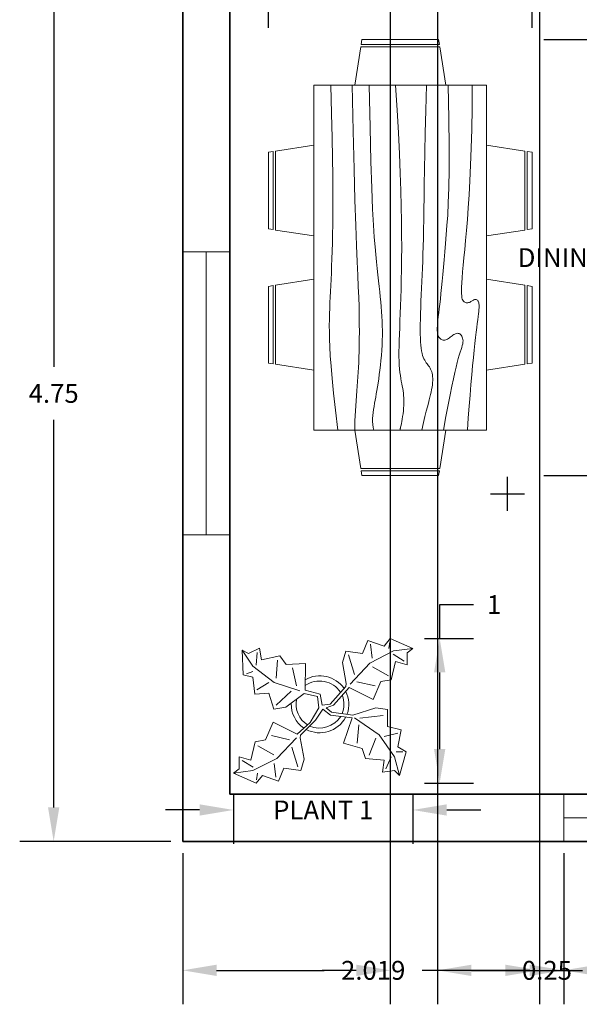
# Model space of a CAD drawing. Units: metres. Extents: x 180.3 to 196.1, y 135.7 to 166.1.
# Tile 1 of 5: x 180.3 to 183.3, y 150.9 to 156.1. Entities that reach past the tile are written whole.
import ezdxf

# ---------------------------------------------------------------- set-up
doc = ezdxf.new("R2010")
doc.units = ezdxf.units.M
doc.header["$MEASUREMENT"] = 0
for name, color, linetype, lineweight in [('A-ANNO-DIMS', 2, 'Continuous', 18), ('A-FURN', 190, 'Continuous', 18), ('A-GLAZ', 130, 'Continuous', 18), ('wall', 50, 'Continuous', 35)]:
    doc.layers.add(name, color=color, linetype=linetype, lineweight=lineweight)
doc.styles.get("Standard").update_dxf_attribs({"font": 'arial.ttf', "height": 0.1})
doc.dimstyles.get("Standard").update_dxf_attribs({"dimtxt": 0.18, "dimasz": 0.18, "dimexe": 0.18, "dimexo": 0.0625, "dimgap": 0.09, "dimtad": 0, "dimtih": 1, "dimtoh": 1, "dimdec": 4, "dimzin": 0, "dimdsep": 46, "dimtxsty": 'Standard', "dimcen": 0.09, "dimadec": 0, "dimazin": 0, "dimtfac": 1, "dimtdec": 4, "dimtofl": 0, "dimtmove": 0, "dimatfit": 3, "dimfxl": 1, "dimtolj": 1, "dimtzin": 0, "dimarcsym": 0})

# ---------------------------------------------------------------- blocks, each defined once
blk = doc.blocks.new('Dining Set - 36 x 72 in.')
for p, q in [((-22, 27.5), (-22.1562, 26.50042)), ((-22, 27.5), (-6, 27.5)), ((-5.8437, 26.49966), (-6, 27.5)), ((6, 27.5), (5.8438, 26.50042)), ((6, 27.5), (22, 27.5)), ((22.1563, 26.49966), (22, 27.5)), ((-22.2343, 26.00059), (-23.4847, 17.99762)), ((-22.2304, 26), (-5.7608, 26)), ((-5.8416, 26.5), (-22.1534, 26.5)), ((-4.5152, 17.99762), (-5.7655, 25.99926)), ((5.7657, 26.00059), (4.5153, 17.99762)), ((5.7696, 26), (22.2392, 26)), ((22.1584, 26.5), (5.8466, 26.5)), ((23.4848, 17.99762), (22.2345, 25.99926)), ((36, 18), (-36, 18)), ((-36, 18), (-36, -18)), ((36, -18), (36, 18)), ((-44.0006, 8.23428), (-35.9976, 9.48474)), ((-44, 8.23041), (-44, -8.23915)), ((44.0006, 8.23428), (35.9976, 9.48474)), ((44, 8.23041), (44, -8.23915)), ((-45.5, 8), (-44.5004, 8.15617)), ((-45.5, 8), (-45.5, -8)), ((-44.5, -8.15843), (-44.5, 8.15338)), ((44.5, -8.15843), (44.5, 8.15338)), ((45.5, 8), (44.5005, 8.15617)), ((45.5, 8), (45.5, -8)), ((-44.4997, -8.15631), (-45.5, -8)), ((44.4997, -8.15631), (45.5, -8)), ((-35.9976, -9.48476), (-43.9993, -8.2345)), ((35.9976, -9.48476), (43.9993, -8.2345)), ((-36, -18), (36, -18)), ((-22.2343, -26.0006), (-23.4847, -17.99762)), ((-4.5152, -17.99762), (-5.7655, -25.99928)), ((5.7657, -26.0006), (4.5153, -17.99762)), ((23.4848, -17.99762), (22.2345, -25.99928)), ((-22.2304, -26), (-5.7608, -26)), ((-22, -27.5), (-22.1562, -26.50044)), ((-5.8416, -26.5), (-22.1534, -26.5)), ((-5.8437, -26.49967), (-6, -27.5)), ((5.7696, -26), (22.2392, -26)), ((6, -27.5), (5.8438, -26.50044)), ((22.1584, -26.5), (5.8466, -26.5)), ((22.1563, -26.49967), (22, -27.5)), ((-22, -27.5), (-6, -27.5)), ((6, -27.5), (22, -27.5))]:
    blk.add_line(p, q)
for points in [[(-36, 15), (-31.1772, 14.97754), (-26.8079, 14.91406), (-22.8538, 14.81543), (-19.276, 14.6875), (-16.0362, 14.53613), (-13.0957, 14.36718), (-10.4159, 14.18652), (-7.9583, 14), (-5.6904, 13.81315), (-3.6035, 13.63021), (-1.6954, 13.45508), (0.0365, 13.29166), (1.5945, 13.14388), (2.9811, 13.01562), (4.1988, 12.9108), (5.25, 12.83333), (6.1393, 12.78613), (6.8802, 12.76823), (7.4883, 12.77767), (7.9792, 12.8125), (8.3685, 12.87077), (8.6719, 12.95052), (8.9049, 13.0498), (9.0833, 13.16666), (9.2205, 13.29899), (9.3216, 13.44401), (9.3895, 13.59879), (9.4271, 13.76041), (9.4373, 13.92594), (9.4232, 14.09245), (9.3875, 14.257), (9.3333, 14.41666), (9.2638, 14.56917), (9.1836, 14.71484), (9.0975, 14.85465), (9.0104, 14.98958), (8.9272, 15.1206), (8.8529, 15.2487), (8.7922, 15.37483), (8.75, 15.5), (8.7305, 15.62467), (8.7344, 15.74739), (8.7617, 15.86621), (8.8125, 15.97916), (8.8867, 16.08431), (8.9844, 16.17968), (9.1055, 16.26334), (9.25, 16.33333), (9.4189, 16.38802), (9.6172, 16.42708), (9.8506, 16.45052), (10.125, 16.45833), (10.4463, 16.45052), (10.8203, 16.42708), (11.2529, 16.38802), (11.75, 16.33333), (12.3184, 16.26318), (12.9694, 16.17838), (13.7151, 16.07991), (14.5677, 15.96875), (15.5395, 15.84586), (16.6426, 15.71224), (17.8893, 15.56884), (19.2917, 15.41666), (20.859, 15.25667), (22.5879, 15.08984), (24.4721, 14.91715), (26.5052, 14.73958), (28.6809, 14.5581), (30.9929, 14.3737), (33.4347, 14.18733), (36, 14)], [(-36, 10), (-28.9766, 10.14274), (-23.1725, 10.20442), (-18.4241, 10.19775), (-14.5677, 10.13541), (-11.4399, 10.03011), (-8.877, 9.89453), (-6.7154, 9.74137), (-4.7917, 9.58333), (-2.9698, 9.43082), (-1.2246, 9.28515), (0.4415, 9.14534), (2.026, 9.01041), (3.5266, 8.87939), (4.9408, 8.7513), (6.266, 8.62516), (7.5, 8.5), (8.6411, 8.37549), (9.6914, 8.2539), (10.6538, 8.13818), (11.5312, 8.03125), (12.3267, 7.93603), (13.043, 7.85547), (13.6831, 7.79248), (14.25, 7.75), (14.7471, 7.7303), (15.1797, 7.73307), (15.5537, 7.75732), (15.875, 7.80208), (16.1494, 7.86637), (16.3828, 7.94922), (16.5811, 8.04964), (16.75, 8.16666), (16.8944, 8.29915), (17.0143, 8.44531), (17.1089, 8.60319), (17.1771, 8.77083), (17.218, 8.94629), (17.2305, 9.1276), (17.2137, 9.31282), (17.1667, 9.5), (17.0895, 9.6875), (16.987, 9.875), (16.8649, 10.0625), (16.7292, 10.25), (16.5856, 10.4375), (16.4401, 10.625), (16.2985, 10.8125), (16.1667, 11), (16.05, 11.18733), (15.9518, 11.3737), (15.8752, 11.5581), (15.8229, 11.73958), (15.798, 11.91715), (15.8034, 12.08984), (15.842, 12.25667), (15.9167, 12.41666), (16.0295, 12.56836), (16.1784, 12.70833), (16.3605, 12.83268), (16.5729, 12.9375), (16.8127, 13.01888), (17.0768, 13.07291), (17.3625, 13.0957), (17.6667, 13.08333), (17.9894, 13.03312), (18.3418, 12.94726), (18.7382, 12.82918), (19.1927, 12.68229), (19.7195, 12.51001), (20.3327, 12.31575), (21.0465, 12.10294), (21.875, 11.875), (22.8357, 11.63354), (23.959, 11.37304), (25.2786, 11.08618), (26.8282, 10.76562), (28.6414, 10.40405), (30.752, 9.99414), (33.1936, 9.52856), (36, 9)], [(-36, 5.5), (-30.7157, 5.3348), (-26.069, 5.20963), (-21.9946, 5.11767), (-18.4271, 5.05208), (-15.3009, 5.00602), (-12.5508, 4.97265), (-10.1112, 4.94515), (-7.9167, 4.91666), (-5.909, 4.88167), (-4.0586, 4.83984), (-2.3429, 4.79215), (-0.7396, 4.73958), (0.7739, 4.6831), (2.22, 4.6237), (3.6213, 4.56233), (5, 4.5), (6.373, 4.43782), (7.7344, 4.3776), (9.0723, 4.32129), (10.375, 4.27083), (11.6309, 4.22819), (12.8281, 4.19531), (13.9551, 4.17415), (15, 4.16666), (15.954, 4.17448), (16.819, 4.19791), (17.6001, 4.23698), (18.3021, 4.29166), (18.9299, 4.36198), (19.4883, 4.44791), (19.9823, 4.54948), (20.4167, 4.66666), (20.7969, 4.79899), (21.1302, 4.94401), (21.4245, 5.09879), (21.6875, 5.26041), (21.9271, 5.42594), (22.1511, 5.59245), (22.3672, 5.757), (22.5834, 5.91666), (22.8065, 6.06868), (23.0404, 6.21093), (23.2879, 6.34147), (23.5521, 6.45833), (23.8358, 6.55957), (24.142, 6.64323), (24.4735, 6.70735), (24.8334, 6.75), (25.2235, 6.76969), (25.642, 6.76692), (26.0858, 6.74267), (26.5521, 6.69791), (27.0379, 6.63362), (27.5404, 6.55078), (28.0565, 6.45036), (28.5834, 6.33333), (29.1242, 6.19987), (29.7071, 6.04687), (30.3661, 5.87044), (31.1354, 5.66666), (32.0493, 5.43164), (33.142, 5.16146), (34.4475, 4.85221), (36, 4.5)], [(-36, -1), (-30.7915, -0.6591), (-26.0195, -0.38216), (-21.6519, -0.16284), (-17.6563, 0.00521), (-14.0005, 0.12833), (-10.6523, 0.21289), (-7.5796, 0.26522), (-4.75, 0.29166), (-2.134, 0.29793), (0.2878, 0.28711), (2.5317, 0.26163), (4.6146, 0.22396), (6.5529, 0.17651), (8.3633, 0.12174), (10.0623, 0.06209), (11.6667, 0), (13.1899, -0.06201), (14.6341, -0.1211), (15.9982, -0.17432), (17.2813, -0.21875), (18.4823, -0.25147), (19.6003, -0.26953), (20.6343, -0.27002), (21.5834, -0.25), (22.4481, -0.20768), (23.2357, -0.14584), (23.9549, -0.06836), (24.6146, 0.02083), (25.2235, 0.11784), (25.7904, 0.21875), (26.3241, 0.31966), (26.8334, 0.41666), (27.3265, 0.50618), (27.8099, 0.58593), (28.2894, 0.65397), (28.7709, 0.70833), (29.2601, 0.74707), (29.763, 0.76823), (30.2855, 0.76985), (30.8334, 0.75), (31.4088, 0.70784), (31.9994, 0.64713), (32.589, 0.57275), (33.1615, 0.48958), (33.7008, 0.4025), (34.1908, 0.3164), (34.6153, 0.23616), (34.9584, 0.16666), (35.2099, 0.11165), (35.3848, 0.07031), (35.504, 0.04069), (35.5886, 0.02083), (35.6594, 0.00879), (35.7377, 0.0026), (35.8442, 0.00032), (36, 0)], [(-36, -6.5), (-27.1843, -6.31267), (-20.084, -6.1263), (-14.469, -5.9419), (-10.1094, -5.76042), (-6.7752, -5.58285), (-4.2363, -5.41016), (-2.2629, -5.24333), (-0.625, -5.08334), (0.8708, -4.93099), (2.2715, -4.78646), (3.5872, -4.64974), (4.8281, -4.52084), (6.0046, -4.39974), (7.127, -4.28646), (8.2053, -4.18099), (9.25, -4.08334), (10.2705, -3.99382), (11.2734, -3.91407), (12.2647, -3.84603), (13.25, -3.79167), (14.2354, -3.75293), (15.2266, -3.73177), (16.2295, -3.73015), (17.25, -3.75), (18.2912, -3.79248), (19.3451, -3.85547), (20.4009, -3.93604), (21.4479, -4.03125), (22.4754, -4.13819), (23.4727, -4.25391), (24.4289, -4.37549), (25.3334, -4.5), (26.1785, -4.62492), (26.9694, -4.74935), (27.7145, -4.87281), (28.4219, -4.99479), (29.1, -5.11483), (29.7572, -5.23242), (30.4016, -5.34709), (31.0417, -5.45834), (31.6837, -5.56437), (32.3262, -5.65821), (32.9658, -5.73153), (33.599, -5.77604), (34.2224, -5.78345), (34.8327, -5.74545), (35.4264, -5.65373), (36, -5.5)], [(-36, -10), (-26.4022, -9.81299), (-18.4675, -9.62891), (-11.9839, -9.45069), (-6.7396, -9.28125), (-2.5226, -9.12354), (0.8789, -8.98047), (3.6769, -8.85498), (6.0833, -8.75), (8.2767, -8.66765), (10.3021, -8.60677), (12.1712, -8.56543), (13.8958, -8.54167), (15.4876, -8.53353), (16.9583, -8.53907), (18.3197, -8.55632), (19.5834, -8.58334), (20.7616, -8.61841), (21.8685, -8.66081), (22.9188, -8.71004), (23.9271, -8.76563), (24.9081, -8.82707), (25.8763, -8.89388), (26.8465, -8.96558), (27.8334, -9.04167), (28.8474, -9.12118), (29.8828, -9.20117), (30.93, -9.27824), (31.9792, -9.34896), (33.0205, -9.40991), (34.0443, -9.45768), (35.0407, -9.48885), (36, -9.5)], [(-36, -14.5), (-30.0881, -14.33513), (-25.0332, -14.21224), (-20.7312, -14.12647), (-17.0781, -14.07292), (-13.97, -14.04671), (-11.3027, -14.04297), (-8.9724, -14.05681), (-6.875, -14.08334), (-4.9224, -14.11833), (-3.0905, -14.16016), (-1.3709, -14.20785), (0.2448, -14.26042), (1.7647, -14.3169), (3.1973, -14.3763), (4.5507, -14.43767), (5.8333, -14.5), (7.0554, -14.5621), (8.235, -14.62175), (9.3922, -14.67652), (10.5469, -14.72396), (11.7192, -14.76164), (12.929, -14.78711), (14.1965, -14.79794), (15.5417, -14.79167), (16.9933, -14.76424), (18.6152, -14.70508), (20.4804, -14.60197), (22.6615, -14.44271), (25.2312, -14.21509), (28.2624, -13.9069), (31.8277, -13.50594), (36, -13)]]:
    blk.add_lwpolyline(points)
blk = doc.blocks.new('Plant - Rubber or Philodendron')
for p, q in [((8.8871, 10.7908), (9.9809, 13.4933)), ((9.9809, 13.4933), (13.3837, 12.301)), ((10.5828, 12.6946), (10.8893, 9.7953)), ((13.3837, 12.301), (14.68, 13.9039)), ((14.5816, 13.2037), (14.3848, 11.8033)), ((14.68, 13.9039), (19.3848, 11.8146)), ((-16.2005, 11.4774), (-13.9899, 8.1064)), ((-16.2005, 11.4774), (-14.8639, 10.7964)), ((-16.0159, 6.3329), (-16.2005, 11.4774)), ((-14.8639, 10.7964), (-12.6195, 11.8975)), ((-13.3174, 8.325), (-13.0735, 11.0065)), ((-12.6195, 11.8975), (-12.1909, 9.4345)), ((-12.1909, 9.4345), (-8.3829, 10.3)), ((-8.3829, 10.3), (-7.0549, 8.501)), ((4.6914, 8.8812), (5.3859, 11.2828)), ((5.3859, 11.2828), (8.8871, 10.7908)), ((5.9878, 10.4842), (7.1971, 6.3869)), ((15.3859, 11.3055), (10.3916, 8.7942)), ((15.2875, 10.6053), (17.5907, 9.2105)), ((19.3848, 11.8146), (15.3859, 11.3055)), ((19.3848, 11.8146), (18.1868, 10.9119)), ((18.1868, 10.9119), (18.1925, 8.4119)), ((-8.8369, 9.409), (-9.0894, 5.6095)), ((-7.0549, 8.501), (-3.0284, 8.6941)), ((-3.0284, 8.6941), (-3.0709, 3.1041)), ((4.6914, 8.8812), (5.5014, 4.4831)), ((10.3916, 8.7942), (6.2847, 4.4028)), ((15.7909, 9.1065), (14.8995, 5.3044)), ((18.1925, 8.4119), (15.7909, 9.1065)), ((-14.0069, 5.8704), (-16.0159, 6.3329)), ((-15.3434, 6.5514), (-13.9984, 6.9884)), ((-13.9899, 8.1064), (-9.5434, 4.7185)), ((-4.8529, 4.012), (-5.7184, 7.82)), ((14.2977, 6.1031), (10.9934, 7.9956)), ((-13.5868, 2.2894), (-14.0069, 5.8704)), ((-13.1329, 3.1804), (-10.6614, 4.727)), ((-9.5434, 4.7185), (-4.1917, 2.9888)), ((5.4346, 3.9146), (5.5014, 4.4831)), ((7.7005, 4.8881), (11.5025, 3.9967)), ((12.7005, 4.8994), (11.1089, 1.1958)), ((14.8995, 5.3044), (12.7005, 4.8994)), ((-10.6784, 2.491), (-13.5868, 2.2894)), ((-9.5858, -0.8715), (-10.6784, 2.491)), ((-9.1318, 0.0195), (-5.9793, 2.9025)), ((-7.1228, -0.443), (-3.5248, 2.2131)), ((-3.5248, 2.2131), (-3.3011, 2.4355)), ((-3.3011, 2.4355), (-0.5306, 1.7947)), ((-3.0709, 3.1041), (0.0797, 2.3163)), ((0.0797, 2.3163), (0.4866, -0.031)), ((2.1141, 0.2298), (5.4346, 3.9146)), ((6.1032, 3.6844), (2.8262, -0.031)), ((11.1089, 1.1958), (6.1032, 3.6844)), ((-0.5306, 1.7947), (-0.2255, -0.5527)), ((-0.5306, 1.7947), (-0.5306, 1.7947)), ((0.4866, -0.031), (2.1141, 0.2298)), ((-7.1228, -0.443), (-9.5858, -0.8715)), ((-2.019, -3.6148), (-0.2255, -0.5527)), ((-0.9375, -3.1608), (0.5883, -0.8135)), ((0.5883, -0.8135), (2.2447, -2.0916)), ((2.8262, -0.031), (1.3003, -0.5527)), ((1.3003, -0.5527), (2.4193, -1.4655)), ((2.4193, -1.4655), (6.895, -2.1175)), ((11.6605, -0.5413), (6.895, -2.1175)), ((11.6605, -0.5413), (14.1354, -0.8948)), ((14.1354, -0.8948), (14.1354, -4.4304)), ((-11.3237, -7.2629), (-9.7321, -3.5593)), ((-9.7321, -3.5593), (-4.7264, -6.0479)), ((-2.019, -3.6148), (-4.7264, -6.0479)), ((-4.0579, -6.2781), (-0.9375, -3.1608)), ((2.2447, -2.0916), (6.7108, -2.6626)), ((4.943, -7.9659), (6.7108, -2.6626)), ((12.3677, -6.1981), (7.219, -2.6772)), ((8.125, -4.0768), (7.7715, -7.9659)), ((8.3544, -2.7453), (13.1973, -2.1704)), ((16.2567, -5.8446), (13.4283, -6.5517)), ((14.1354, -4.4304), (16.9638, -5.1375)), ((16.9638, -5.1375), (16.2567, -8.673)), ((-14.4141, -11.4699), (-13.5228, -7.6679)), ((-13.5228, -7.6679), (-11.3237, -7.2629)), ((-6.3237, -7.2516), (-10.1257, -6.3602)), ((-9.0148, -11.1577), (-4.9047, -6.8122)), ((-4.1246, -6.8466), (-4.0579, -6.2781)), ((-3.3146, -11.2447), (-4.1246, -6.8466)), ((8.8321, -9.0266), (4.943, -7.9659)), ((10.2463, -10.4408), (11.6605, -6.9053)), ((15.5496, -10.7943), (12.3677, -6.1981)), ((-12.921, -8.4665), (-9.6166, -10.359)), ((-4.611, -12.8477), (-5.8203, -8.7504)), ((9.5392, -11.1479), (8.8321, -9.0266)), ((17.3174, -9.7337), (15.9032, -9.7337)), ((16.2567, -8.673), (18.0245, -9.7337)), ((18.0245, -9.7337), (16.6103, -14.6834)), ((-16.8157, -10.7754), (-14.4141, -11.4699)), ((-16.8101, -13.2754), (-16.8157, -10.7754)), ((-13.9107, -12.9688), (-16.2139, -11.574)), ((-14.0091, -13.669), (-9.0148, -11.1577)), ((-9.206, -15.0581), (-9.5126, -12.1588)), ((-3.3146, -11.2447), (-4.0092, -13.6463)), ((13.4283, -11.5015), (9.5392, -11.1479)), ((13.0748, -13.9763), (13.4283, -11.5015)), ((14.8425, -10.7943), (13.7819, -13.2692)), ((16.6103, -14.6834), (15.5496, -10.7943)), ((-18.008, -14.1781), (-16.8101, -13.2754)), ((-18.008, -14.1781), (-14.0091, -13.669)), ((-13.3032, -16.2674), (-18.008, -14.1781)), ((-13.2048, -15.5672), (-13.008, -14.1668)), ((-7.5103, -13.1543), (-8.6042, -15.8568)), ((-4.0092, -13.6463), (-7.5103, -13.1543)), ((15.5496, -13.6228), (13.0748, -13.9763)), ((16.6103, -14.6834), (15.5496, -13.6228)), ((-12.0069, -14.6645), (-13.3032, -16.2674)), ((-8.6042, -15.8568), (-12.0069, -14.6645))]:
    blk.add_line(p, q)
for centre, radius, start, end in [((0, 0), 6.1275, 34.37569, 120.1028), ((-0.0601, -0.2075), 5.2461, 33.82192, 124.9414), ((-0.098, 0.1364), 6.1288, 341.2017, 26.09184), ((0.0308, 0.1664), 6, 178.6147, 235.1169), ((0.0308, 0.1664), 5, 168.1647, 238.6725), ((-0.2664, 0.1682), 5.2775, 338.4094, 20.03007), ((-0.0234, 0.3825), 6.1492, 242.5812, 331.2714), ((-0.1102, 0.4886), 5.2883, 247.3711, 327.472)]:
    blk.add_arc(centre, radius, start, end)
blk = doc.blocks.new('WIN-1500')
for p, q in [((0.0003, 0.2499), (0.0003, -0.0001)), ((1.5003, 0.2499), (1.5003, -0.0001)), ((1.5003, 0.1249), (0.0003, 0.1249))]:
    blk.add_line(p, q)
blk = doc.blocks.new('*D25')
at = {"layer": 'A-ANNO-DIMS', "color": 0, "lineweight": -2, "transparency": 16777216}
for p, q in [((183.1113, 155.9984), (183.5755, 155.9984)), ((183.3955, 155.8184), (183.3955, 154.9844)), ((183.3955, 153.867), (183.3955, 154.701)), ((183.1113, 153.687), (183.5755, 153.687))]:
    blk.add_line(p, q, dxfattribs=at)
at = {"layer": 'A-ANNO-DIMS', "color": 0, "transparency": 16777216}
for points in [[(183.3655, 155.8184), (183.4255, 155.8184), (183.3955, 155.9984)], [(183.3655, 153.867), (183.4255, 153.867), (183.3955, 153.687)]]:
    blk.add_solid(points, dxfattribs=at)
at = {"layer": 'Defpoints', "color": 0, "transparency": 16777216}
for p in [(183.0488, 155.9984), (183.0488, 153.687), (183.3955, 153.687)]:
    blk.add_point(p, dxfattribs=at)
at = {"layer": 'A-ANNO-DIMS', "color": 0, "transparency": 16777216, "insert": (183.3955, 154.8427), "char_height": 0.1, "attachment_point": 5}
blk.add_mtext('\\A1;DINING SET 2', dxfattribs=at)
blk = doc.blocks.new('*D26')
at = {"layer": 'A-ANNO-DIMS', "color": 0, "lineweight": -2, "transparency": 16777216}
for p, q in [((181.6518, 156.0609), (181.6518, 156.5251)), ((183.0488, 156.0609), (183.0488, 156.5251)), ((181.8318, 156.3451), (182.2419, 156.3451)), ((182.8688, 156.3451), (182.4587, 156.3451))]:
    blk.add_line(p, q, dxfattribs=at)
at = {"layer": 'A-ANNO-DIMS', "color": 0, "transparency": 16777216}
for points in [[(181.8318, 156.3751), (181.8318, 156.3151), (181.6518, 156.3451)], [(182.8688, 156.3751), (182.8688, 156.3151), (183.0488, 156.3451)]]:
    blk.add_solid(points, dxfattribs=at)
at = {"layer": 'Defpoints', "color": 0, "transparency": 16777216}
for p in [(183.0488, 156.3451), (181.6518, 155.9984), (183.0488, 155.9984)]:
    blk.add_point(p, dxfattribs=at)
at = {"layer": 'A-ANNO-DIMS', "color": 0, "transparency": 16777216, "insert": (182.3503, 156.3451), "char_height": 0.1, "attachment_point": 5}
blk.add_mtext('\\A1;1', dxfattribs=at)
blk = doc.blocks.new('*D31')
at = {"layer": 'A-ANNO-DIMS', "color": 0, "lineweight": -2, "transparency": 16777216}
for p, q in [((181.467, 151.9945), (181.467, 151.7345)), ((182.4168, 151.9945), (182.4168, 151.7345)), ((181.287, 151.9145), (181.107, 151.9145)), ((182.5968, 151.9145), (182.7768, 151.9145))]:
    blk.add_line(p, q, dxfattribs=at)
at = {"layer": 'A-ANNO-DIMS', "color": 0, "transparency": 16777216}
for points in [[(181.287, 151.9445), (181.287, 151.8845), (181.467, 151.9145)], [(182.5968, 151.9445), (182.5968, 151.8845), (182.4168, 151.9145)]]:
    blk.add_solid(points, dxfattribs=at)
at = {"layer": 'Defpoints', "color": 0, "transparency": 16777216}
for p in [(181.467, 152.057), (182.4168, 152.057), (182.4168, 151.9145)]:
    blk.add_point(p, dxfattribs=at)
at = {"layer": 'A-ANNO-DIMS', "color": 0, "transparency": 16777216, "insert": (181.9419, 151.9145), "char_height": 0.1, "attachment_point": 5}
blk.add_mtext('\\A1;PLANT 1', dxfattribs=at)
blk = doc.blocks.new('*D32')
at = {"layer": 'A-ANNO-DIMS', "color": 0, "lineweight": -2, "transparency": 16777216}
for p, q in [((182.5592, 152.8233), (182.5592, 153.0033)), ((182.5592, 153.0033), (182.7392, 153.0033)), ((182.4793, 152.8233), (182.7392, 152.8233)), ((182.5592, 152.237), (182.5592, 152.6433)), ((182.4793, 152.057), (182.7392, 152.057))]:
    blk.add_line(p, q, dxfattribs=at)
at = {"layer": 'A-ANNO-DIMS', "color": 0, "transparency": 16777216}
for points in [[(182.5292, 152.6433), (182.5892, 152.6433), (182.5592, 152.8233)], [(182.5292, 152.237), (182.5892, 152.237), (182.5592, 152.057)]]:
    blk.add_solid(points, dxfattribs=at)
at = {"layer": 'Defpoints', "color": 0, "transparency": 16777216}
for p in [(182.4168, 152.8233), (182.5592, 152.8233), (182.4168, 152.057)]:
    blk.add_point(p, dxfattribs=at)
at = {"layer": 'A-ANNO-DIMS', "color": 0, "transparency": 16777216, "insert": (182.8477, 153.0033), "char_height": 0.1, "attachment_point": 5}
blk.add_mtext('\\A1;1', dxfattribs=at)
blk = doc.blocks.new('*D36')
at = {"layer": 'A-ANNO-DIMS', "color": 0, "lineweight": -2, "transparency": 16777216}
for p, q in [((181.1348, 156.4979), (180.3336, 156.4979)), ((180.5136, 156.3179), (180.5136, 154.2638)), ((180.5136, 151.9279), (180.5136, 153.982)), ((181.1348, 151.7479), (180.3336, 151.7479))]:
    blk.add_line(p, q, dxfattribs=at)
at = {"layer": 'A-ANNO-DIMS', "color": 0, "transparency": 16777216}
for points in [[(180.4836, 156.3179), (180.5436, 156.3179), (180.5136, 156.4979)], [(180.4836, 151.9279), (180.5436, 151.9279), (180.5136, 151.7479)]]:
    blk.add_solid(points, dxfattribs=at)
at = {"layer": 'Defpoints', "color": 0, "transparency": 16777216}
for p in [(180.5136, 156.4979), (181.1973, 156.4979), (181.1973, 151.7479)]:
    blk.add_point(p, dxfattribs=at)
at = {"layer": 'A-ANNO-DIMS', "color": 0, "transparency": 16777216, "insert": (180.5136, 154.1229), "char_height": 0.1, "attachment_point": 5}
blk.add_mtext('\\A1;4.75', dxfattribs=at)
blk = doc.blocks.new('*D39')
at = {"layer": 'A-ANNO-DIMS', "color": 0, "lineweight": -2, "transparency": 16777216}
for p, q in [((181.1973, 151.6854), (181.1973, 150.8842)), ((183.2164, 151.6854), (183.2164, 150.8842)), ((181.3773, 151.0642), (181.9472, 151.0642)), ((183.0364, 151.0642), (182.4665, 151.0642))]:
    blk.add_line(p, q, dxfattribs=at)
at = {"layer": 'A-ANNO-DIMS', "color": 0, "transparency": 16777216}
for points in [[(181.3773, 151.0942), (181.3773, 151.0342), (181.1973, 151.0642)], [(183.0364, 151.0942), (183.0364, 151.0342), (183.2164, 151.0642)]]:
    blk.add_solid(points, dxfattribs=at)
at = {"layer": 'Defpoints', "color": 0, "transparency": 16777216}
for p in [(181.1973, 151.7479), (183.2164, 151.7479), (183.2164, 151.0642)]:
    blk.add_point(p, dxfattribs=at)
at = {"layer": 'A-ANNO-DIMS', "color": 0, "transparency": 16777216, "insert": (182.2069, 151.0642), "char_height": 0.1, "attachment_point": 5}
blk.add_mtext('\\A1;2.019', dxfattribs=at)
blk = doc.blocks.new('*D40')
at = {"layer": 'A-ANNO-DIMS', "color": 0, "lineweight": -2, "transparency": 16777216}
for p, q in [((183.2164, 151.6854), (183.2164, 150.8842)), ((184.7164, 151.6854), (184.7164, 150.8842)), ((183.3964, 151.0642), (183.7897, 151.0642)), ((184.5364, 151.0642), (184.1431, 151.0642))]:
    blk.add_line(p, q, dxfattribs=at)
at = {"layer": 'A-ANNO-DIMS', "color": 0, "transparency": 16777216}
for points in [[(183.3964, 151.0942), (183.3964, 151.0342), (183.2164, 151.0642)], [(184.5364, 151.0942), (184.5364, 151.0342), (184.7164, 151.0642)]]:
    blk.add_solid(points, dxfattribs=at)
at = {"layer": 'Defpoints', "color": 0, "transparency": 16777216}
for p in [(183.2164, 151.7479), (184.7164, 151.7479), (184.7164, 151.0642)]:
    blk.add_point(p, dxfattribs=at)
at = {"layer": 'A-ANNO-DIMS', "color": 0, "transparency": 16777216, "insert": (183.9664, 151.0642), "char_height": 0.1, "attachment_point": 5}
blk.add_mtext('\\A1;1.5', dxfattribs=at)
blk = doc.blocks.new('*D50')
at = {"layer": 'A-ANNO-DIMS', "color": 0, "lineweight": -2, "transparency": 16777216}
for p, q in [((182.2973, 156.4354), (182.2973, 150.8842)), ((182.5473, 156.4354), (182.5473, 150.8842)), ((182.1173, 151.0642), (181.9373, 151.0642)), ((182.7273, 151.0642), (182.9073, 151.0642))]:
    blk.add_line(p, q, dxfattribs=at)
at = {"layer": 'A-ANNO-DIMS', "color": 0, "transparency": 16777216}
for points in [[(182.1173, 151.0942), (182.1173, 151.0342), (182.2973, 151.0642)], [(182.7273, 151.0942), (182.7273, 151.0342), (182.5473, 151.0642)]]:
    blk.add_solid(points, dxfattribs=at)
at = {"layer": 'Defpoints', "color": 0, "transparency": 16777216}
for p in [(182.2973, 156.4979), (182.5473, 156.4979), (182.5473, 151.0642)]:
    blk.add_point(p, dxfattribs=at)
at = {"layer": 'A-ANNO-DIMS', "color": 0, "transparency": 16777216, "insert": (183.1276, 151.0642), "char_height": 0.1, "attachment_point": 5}
blk.add_mtext('\\A1;0.25', dxfattribs=at)
blk = doc.blocks.new('*D51')
at = {"layer": 'A-ANNO-DIMS', "color": 0, "lineweight": -2, "transparency": 16777216}
for p, q in [((182.5473, 156.4354), (182.5473, 150.8842)), ((183.0878, 156.4354), (183.0878, 150.8842)), ((182.7273, 151.0642), (182.9078, 151.0642)), ((183.0878, 151.0642), (183.2678, 151.0642))]:
    blk.add_line(p, q, dxfattribs=at)
at = {"layer": 'A-ANNO-DIMS', "color": 0, "transparency": 16777216}
for points in [[(182.7273, 151.0942), (182.7273, 151.0342), (182.5473, 151.0642)], [(182.9078, 151.0942), (182.9078, 151.0342), (183.0878, 151.0642)]]:
    blk.add_solid(points, dxfattribs=at)
at = {"layer": 'Defpoints', "color": 0, "transparency": 16777216}
for p in [(182.5473, 156.4979), (183.0878, 156.4979), (183.0878, 151.0642)]:
    blk.add_point(p, dxfattribs=at)
at = {"layer": 'A-ANNO-DIMS', "color": 0, "transparency": 16777216, "insert": (183.4875, 151.0642), "char_height": 0.1, "attachment_point": 5}
blk.add_mtext('\\A1;0.54', dxfattribs=at)
blk = doc.blocks.new('*D52')
at = {"layer": 'A-ANNO-DIMS', "color": 0, "lineweight": -2, "transparency": 16777216}
for p, q in [((182.5473, 158.3772), (182.5473, 150.8842)), ((184.5151, 158.3772), (184.5151, 150.8842)), ((182.7273, 151.0642), (183.316, 151.0642)), ((184.3351, 151.0642), (183.7464, 151.0642))]:
    blk.add_line(p, q, dxfattribs=at)
at = {"layer": 'A-ANNO-DIMS', "color": 0, "transparency": 16777216}
for points in [[(182.7273, 151.0942), (182.7273, 151.0342), (182.5473, 151.0642)], [(184.3351, 151.0942), (184.3351, 151.0342), (184.5151, 151.0642)]]:
    blk.add_solid(points, dxfattribs=at)
at = {"layer": 'Defpoints', "color": 0, "transparency": 16777216}
for p in [(182.5473, 158.4397), (184.5151, 158.4397), (184.5151, 151.0642)]:
    blk.add_point(p, dxfattribs=at)
at = {"layer": 'A-ANNO-DIMS', "color": 0, "transparency": 16777216, "insert": (183.5312, 151.0642), "char_height": 0.1, "attachment_point": 5}
blk.add_mtext('\\A1;1.97', dxfattribs=at)
blk = doc.blocks.new('*D69')
at = {"layer": 'A-ANNO-DIMS', "color": 0, "lineweight": -2, "transparency": 16777216}
for p, q in [((182.9181, 153.5006), (182.9181, 153.6806)), ((182.8281, 153.5906), (183.0081, 153.5906)), ((184.4065, 153.5912), (184.0284, 153.5911))]:
    blk.add_line(p, q, dxfattribs=at)
at = {"layer": 'A-ANNO-DIMS', "color": 0, "transparency": 16777216}
blk.add_solid([(184.0284, 153.6211), (184.0284, 153.5611), (183.8484, 153.591)], dxfattribs=at)
at = {"layer": 'Defpoints', "color": 0, "transparency": 16777216}
for p in [(182.9181, 153.5906), (183.8484, 153.591)]:
    blk.add_point(p, dxfattribs=at)
at = {"layer": 'A-ANNO-DIMS', "color": 0, "transparency": 16777216, "insert": (184.7826, 153.5912), "char_height": 0.1, "attachment_point": 5}
blk.add_mtext('\\A1;2X R0.93', dxfattribs=at)

msp = doc.modelspace()

# ---------------------------------------------------------------- linework, layer by layer
at = {"layer": 'wall'}
for p, q in [((181.1973, 156.4979), (181.1973, 151.7479)), ((181.4473, 156.2479), (181.4473, 151.9979)), ((186.8354, 151.9979), (181.4473, 151.9979)), ((186.7354, 151.7479), (181.1973, 151.7479))]:
    msp.add_line(p, q, dxfattribs=at)

# ---------------------------------------------------------------- block references
at = {"layer": 'A-FURN', "xscale": 0.0254, "yscale": 0.0254, "zscale": 0.0254, "rotation": 270}
msp.add_blockref('Dining Set - 36 x 72 in.', (182.3503, 154.8427), dxfattribs=at)
at = {"layer": 'A-FURN', "xscale": 0.0254, "yscale": 0.0254, "zscale": 0.0254}
msp.add_blockref('Plant - Rubber or Philodendron', (181.9244, 152.4702), dxfattribs=at)
at = {"layer": 'A-GLAZ', "rotation": 90.00000000000104}
msp.add_blockref('WIN-1500', (181.4472, 153.3726), dxfattribs=at)
at = {"layer": 'A-GLAZ'}
msp.add_blockref('WIN-1500', (183.216, 151.748), dxfattribs=at)

# ---------------------------------------------------------------- dimensions: what is measured, and where the dimension line sits
at = {"layer": 'A-ANNO-DIMS'}
for base, p1, p2, override, picture, middle in [((184.5151, 151.0642), (182.5473, 158.4397), (184.5151, 158.4397), {"dimdec": 2, "dimlfac": 1, "dimrnd": 0, "dimzin": 0, "dimdsep": 46, "dimlunit": 2}, '*D52', (183.5312, 151.0642)), ((183.0488, 156.3451), (181.6518, 155.9984), (183.0488, 155.9984), {"dimdec": 0, "dimlfac": 1, "dimrnd": 0, "dimzin": 0, "dimdsep": 46, "dimlunit": 2}, '*D26', (182.3503, 156.3451)), ((182.5473, 151.0642), (182.2973, 156.4979), (182.5473, 156.4979), {"dimdec": 2, "dimlfac": 1, "dimrnd": 0, "dimzin": 0, "dimdsep": 46, "dimlunit": 2}, '*D50', (183.1276, 151.0642)), ((183.0878, 151.0642), (182.5473, 156.4979), (183.0878, 156.4979), {"dimdec": 2, "dimlfac": 1, "dimrnd": 0, "dimzin": 0, "dimdsep": 46, "dimlunit": 2}, '*D51', (183.4875, 151.0642)), ((183.2164, 151.0642), (181.1973, 151.7479), (183.2164, 151.7479), {"dimdec": 3, "dimlfac": 1, "dimrnd": 0, "dimzin": 0, "dimdsep": 46, "dimlunit": 2}, '*D39', (182.2069, 151.0642)), ((184.7164, 151.0642), (183.2164, 151.7479), (184.7164, 151.7479), {"dimdec": 1, "dimlfac": 1, "dimrnd": 0, "dimzin": 0, "dimdsep": 46, "dimlunit": 2}, '*D40', (183.9664, 151.0642))]:
    dim = msp.add_linear_dim(base=base, p1=p1, p2=p2, dimstyle='Standard', override=override, dxfattribs=at)
    dim.commit()
    dim.dimension.update_dxf_attribs({"geometry": picture, "text_midpoint": middle})
for base, p1, p2, override, picture, middle in [((180.5136, 156.4979), (181.1973, 151.7479), (181.1973, 156.4979), {"dimdec": 2, "dimlfac": 1, "dimrnd": 0, "dimzin": 0, "dimdsep": 46, "dimlunit": 2}, '*D36', (180.5136, 154.1229)), ((182.5592, 152.8233), (182.4168, 152.057), (182.4168, 152.8233), {"dimdec": 0, "dimlfac": 1, "dimrnd": 0, "dimzin": 0, "dimdsep": 46, "dimlunit": 2}, '*D32', (182.8477, 153.0033))]:
    dim = msp.add_linear_dim(base=base, p1=p1, p2=p2, angle=90, dimstyle='Standard', override=override, dxfattribs=at)
    dim.commit()
    dim.dimension.update_dxf_attribs({"geometry": picture, "text_midpoint": middle})
dim = msp.add_linear_dim(base=(183.3955, 153.687), p1=(183.0488, 155.9984), p2=(183.0488, 153.687), angle=270, text='DINING SET <>', dimstyle='Standard', override={"dimdec": 0, "dimlfac": 1, "dimrnd": 0, "dimzin": 0, "dimdsep": 46, "dimlunit": 2}, dxfattribs=at)
dim.commit()
dim.dimension.update_dxf_attribs({"geometry": '*D25', "text_midpoint": (183.3955, 154.8427)})
dim = msp.add_radius_dim(center=(182.9181, 153.5906), mpoint=(183.8484, 153.591), text='2X <>', dimstyle='Standard', override={"dimdec": 2, "dimlfac": 1, "dimrnd": 0, "dimzin": 0, "dimdsep": 46, "dimlunit": 2}, dxfattribs=at)
dim.commit()
dim.dimension.update_dxf_attribs({"geometry": '*D69', "text_midpoint": (184.4065, 153.5912), "dimtype": 164})
dim = msp.add_linear_dim(base=(182.4168, 151.9145), p1=(181.467, 152.057), p2=(182.4168, 152.057), text='PLANT <>', dimstyle='Standard', override={"dimdec": 0, "dimlfac": 1, "dimrnd": 0, "dimzin": 0, "dimdsep": 46, "dimlunit": 2}, dxfattribs=at)
dim.commit()
dim.dimension.update_dxf_attribs({"geometry": '*D31', "text_midpoint": (181.9419, 151.9145)})

doc.saveas('drawing.dxf')
